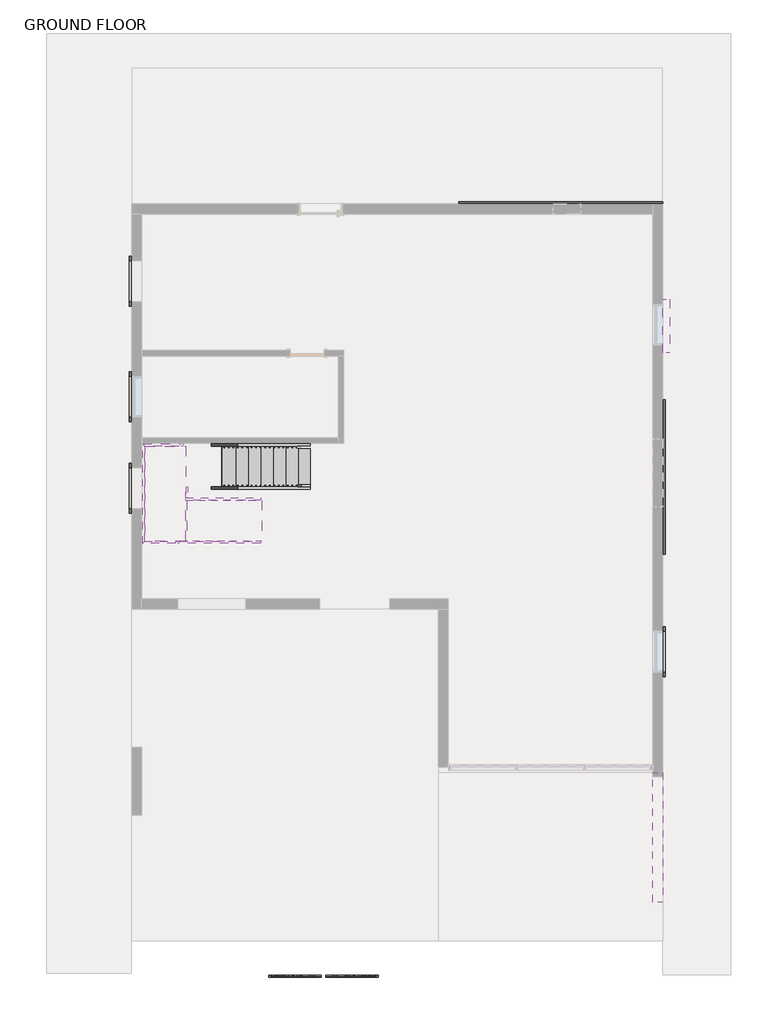
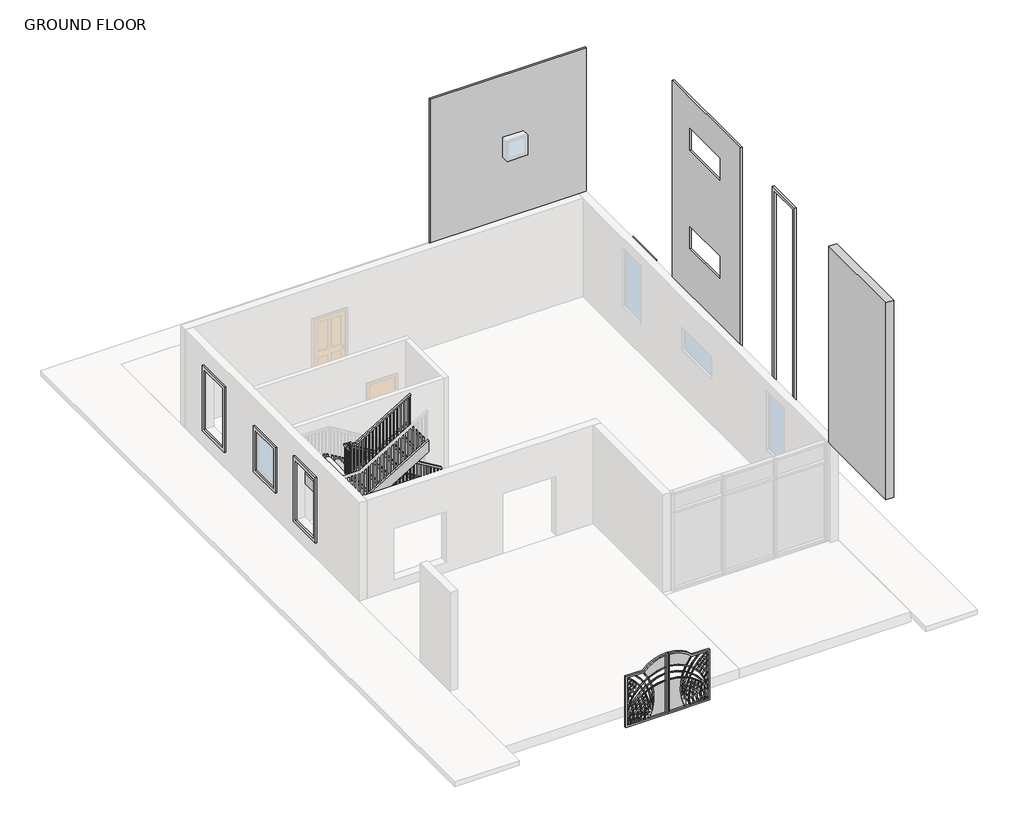
# One storey, part 3 of 3: 9 proxies, 8 members, 2 stair flights, 1 railing, 1 slab.
"""IFC4 building model written with IfcOpenShell, lengths in millimetres."""

from ifc_helpers import new_model, si_unit, frame, origin, place, context, project, spatial, polyline, outline, extrude, faceted_brep, transform, mapped, element, save
from components import generic_models_1_generic_models_1_1482fe98, generic_models_13_generic_models_13_61cfa3f2, generic_models_14_generic_models_13_4ffb657b, generic_models_17_generic_models_17_cb6d61f1, generic_models_20_generic_models_20_543834f7, generic_models_21_generic_models_23_029173b4, generic_models_24_generic_models_24_8205a677, gate_7956_gate_7956_6bc30956, non_monolithic_landing_459b2879, stair_flight_26c172ca, stair_flight_86d1b198

model = new_model("IFC4")

# Units and contexts
model_context = context("Model", 3, world=origin())
ifc_project = project(units=[si_unit("LENGTHUNIT", "METRE", prefix="MILLI")], contexts=[model_context])

# Site, building, storey
site = spatial("IfcSite", under=ifc_project)
building = spatial("IfcBuilding", under=site)
storey = spatial("IfcBuildingStorey", under=building, Name="GROUND FLOOR", Elevation=304.8)

# Proxies
placement = place(None, origin())
generic_models_1_generic_models_1_shape = generic_models_1_generic_models_1_1482fe98(model_context)
element("IfcBuildingElementProxy", 1, Name="Generic Models 1 : Generic Models 1", ObjectType="Generic Models 1 : Generic Models 1", at=placement, inside=storey, context=model_context, shape_type="MappedRepresentation", body=[
    mapped(generic_models_1_generic_models_1_shape, transform((0.0, 0.0, 0.0), x_axis=(1.0, 0.0, 0.0), y_axis=(0.0, 1.0, 0.0), z_axis=(0.0, 0.0, 1.0))),
])
generic_models_13_generic_models_13_shape = generic_models_13_generic_models_13_61cfa3f2(model_context)
element("IfcBuildingElementProxy", 2, Name="Generic Models 13 : Generic Models 13", ObjectType="Generic Models 13 : Generic Models 13", at=placement, inside=storey, context=model_context, shape_type="MappedRepresentation", body=[
    mapped(generic_models_13_generic_models_13_shape, transform((0.0, 0.0, 0.0), x_axis=(1.0, 0.0, 0.0), y_axis=(0.0, 1.0, 0.0), z_axis=(0.0, 0.0, 1.0))),
])
generic_models_14_generic_models_13_shape = generic_models_14_generic_models_13_4ffb657b(model_context)
element("IfcBuildingElementProxy", 3, Name="Generic Models 16 : Generic Models 13", ObjectType="Generic Models 16 : Generic Models 13", at=placement, inside=storey, context=model_context, shape_type="MappedRepresentation", body=[
    mapped(generic_models_14_generic_models_13_shape, transform((0.0, 7315.2, -6096.0), x_axis=(1.0, 0.0, 0.0), y_axis=(0.0, 1.0, 0.0), z_axis=(0.0, 0.0, 1.0))),
])
generic_models_17_generic_models_17_shape = generic_models_17_generic_models_17_cb6d61f1(model_context)
element("IfcBuildingElementProxy", 4, Name="Generic Models 17 : Generic Models 17", ObjectType="Generic Models 17 : Generic Models 17", at=placement, inside=storey, context=model_context, shape_type="MappedRepresentation", body=[
    mapped(generic_models_17_generic_models_17_shape, transform((0.0, 0.0, 0.0), x_axis=(1.0, 0.0, 0.0), y_axis=(0.0, 1.0, 0.0), z_axis=(0.0, 0.0, 1.0))),
])
generic_models_20_generic_models_20_shape = generic_models_20_generic_models_20_543834f7(model_context)
element("IfcBuildingElementProxy", 5, Name="Generic Models 20 : Generic Models 20", ObjectType="Generic Models 20 : Generic Models 20", at=placement, inside=storey, context=model_context, shape_type="MappedRepresentation", body=[
    mapped(generic_models_20_generic_models_20_shape, transform((0.0, 0.0, 0.0), x_axis=(1.0, 0.0, 0.0), y_axis=(0.0, 1.0, 0.0), z_axis=(0.0, 0.0, 1.0))),
])
generic_models_21_generic_models_23_shape = generic_models_21_generic_models_23_029173b4(model_context)
element("IfcBuildingElementProxy", 6, Name="Generic Models 22 : Generic Models 23", ObjectType="Generic Models 22 : Generic Models 23", at=placement, inside=storey, context=model_context, shape_type="MappedRepresentation", body=[
    mapped(generic_models_21_generic_models_23_shape, transform((0.0, 0.0, -6400.8), x_axis=(1.0, 0.0, 0.0), y_axis=(0.0, 1.0, 0.0), z_axis=(0.0, 0.0, 1.0))),
])
generic_models_24_generic_models_24_shape = generic_models_24_generic_models_24_8205a677(model_context)
element("IfcBuildingElementProxy", 7, Name="Generic Models 26 : Generic Models 24", ObjectType="Generic Models 26 : Generic Models 24", at=placement, inside=storey, context=model_context, shape_type="MappedRepresentation", body=[
    mapped(generic_models_24_generic_models_24_shape, transform((0.0, 0.0, -6096.0), x_axis=(1.0, 0.0, 0.0), y_axis=(0.0, 1.0, 0.0), z_axis=(0.0, 0.0, 1.0))),
])
element("IfcBuildingElementProxy", 8, Name="Generic Models 29 : Generic Models 23", ObjectType="Generic Models 29 : Generic Models 23", at=placement, inside=storey, context=model_context, shape_type="MappedRepresentation", body=[
    mapped(generic_models_21_generic_models_23_shape, transform((0.0, -4635.5, -6400.8), x_axis=(1.0, 0.0, 0.0), y_axis=(0.0, 1.0, 0.0), z_axis=(0.0, 0.0, 1.0))),
])
gate_7956_gate_7956_shape = gate_7956_gate_7956_6bc30956(model_context)
element("IfcBuildingElementProxy", 9, Name="gate_7956 : gate_7956", ObjectType="gate_7956 : gate_7956", at=placement, inside=storey, context=model_context, shape_type="MappedRepresentation", body=[
    mapped(gate_7956_gate_7956_shape, transform((-5706.3281265, -8922.5779205, 304.8), x_axis=(1.0, 0.0, 0.0), y_axis=(0.0, 1.0, 0.0), z_axis=(0.0, 0.0, 1.0))),
])

# Members
element("IfcMember", 10, ObjectType="Stringer - 2\" Width", at=placement, inside=storey, context=model_context, shape_type="SweptSolid", body=[
    extrude(outline(polyline([(304.8, -5990.8517085), (516.914512, -5990.8517085), (2179.4599665, -8734.0517085), (1823.051205, -8734.0517085), (304.8, -6228.9372203), (304.8, -5990.8517085)])), frame((0.0, 1953.8826226, 0.0), z_axis=(0.0, 1.0, 0.0), x_axis=(0.0, 0.0, 1.0)), (0.0, 0.0, 1.0), 50.8),
])
element("IfcMember", 11, ObjectType="Stringer - 2\" Width", at=placement, inside=storey, context=model_context, shape_type="SweptSolid", body=[
    extrude(outline(polyline([(304.8, -5990.8517085), (516.914512, -5990.8517085), (2243.6666667, -8839.9927638), (1938.8666667, -8925.1472203), (304.8, -6228.9372203), (304.8, -5990.8517085)])), frame((0.0, 2919.0826226, 0.0), z_axis=(0.0, 1.0, 0.0), x_axis=(0.0, 0.0, 1.0)), (0.0, 0.0, 1.0), 50.8),
])
element("IfcMember", 12, ObjectType="Stringer - 2\" Width", at=placement, inside=storey, context=model_context, shape_type="SweptSolid", body=[
    extrude(outline(polyline([(2379.5811786, -8784.8517085), (2023.1724171, -8784.8517085), (3039.1724171, -7108.4517085), (3395.5811786, -7108.4517085), (2379.5811786, -8784.8517085)])), frame((0.0, 1706.4165128, 0.0), z_axis=(0.0, 1.0, 0.0), x_axis=(0.0, 0.0, 1.0)), (0.0, 0.0, 1.0), 50.8),
])
element("IfcMember", 13, ObjectType="Stringer - 2\" Width", at=placement, inside=storey, context=model_context, shape_type="SweptSolid", body=[
    extrude(outline(polyline([(2243.6666667, -9009.1106533), (1938.8666667, -8923.9561967), (3039.1724171, -7108.4517085), (3395.5811786, -7108.4517085), (2243.6666667, -9009.1106533)])), frame((0.0, 741.2165128, 0.0), z_axis=(0.0, 1.0, 0.0), x_axis=(0.0, 0.0, 1.0)), (0.0, 0.0, 1.0), 50.8),
])
element("IfcMember", 14, ObjectType="Stringer - 2\" Width", at=placement, inside=storey, context=model_context, shape_type="SweptSolid", body=[
    extrude(outline(polyline([(-8734.0517085, 1757.2165128), (-8784.8517085, 1757.2165128), (-8784.8517085, 2004.6826226), (-8734.0517085, 2004.6826226), (-8734.0517085, 1757.2165128)])), frame((0.0, 0.0, 1938.8666667), z_axis=(0.0, 0.0, 1.0), x_axis=(1.0, 0.0, 0.0)), (0.0, 0.0, 1.0), 304.8),
])
element("IfcMember", 15, ObjectType="Stringer - 2\" Width", at=placement, inside=storey, context=model_context, shape_type="Brep", body=[
    faceted_brep([(-8839.9927638, 2919.0826226, 2243.6666667), (-8839.9927638, 2969.8826226, 2243.6666667), (-9750.0517085, 2969.8826226, 2243.6666667), (-9699.2517085, 2919.0826226, 2243.6666667), (-8925.1472203, 2919.0826226, 1938.8666667), (-9699.2517085, 2919.0826226, 1938.8666667), (-8925.1472203, 2969.8826226, 1938.8666667), (-9750.0517085, 2969.8826226, 1938.8666667)], [[[0, 1, 2, 3]], [[4, 0, 3, 5]], [[6, 4, 5, 7]], [[1, 6, 7, 2]], [[1, 0, 4, 6]], [[2, 7, 5, 3]]]),
])
element("IfcMember", 16, ObjectType="Stringer - 2\" Width", at=placement, inside=storey, context=model_context, shape_type="SweptSolid", body=[
    extrude(outline(polyline([(-9750.0517085, 2969.8826226), (-9699.2517085, 2919.0826226), (-9699.2517085, 792.0165128), (-9750.0517085, 741.2165128), (-9750.0517085, 2969.8826226)])), frame((0.0, 0.0, 1938.8666667), z_axis=(0.0, 0.0, 1.0), x_axis=(1.0, 0.0, 0.0)), (0.0, 0.0, 1.0), 304.8),
])
element("IfcMember", 17, ObjectType="Stringer - 2\" Width", at=placement, inside=storey, context=model_context, shape_type="Brep", body=[
    faceted_brep([(-9699.2517085, 792.0165128, 2243.6666667), (-9750.0517085, 741.2165128, 2243.6666667), (-9009.1106533, 741.2165128, 2243.6666667), (-9009.1106533, 792.0165128, 2243.6666667), (-9699.2517085, 792.0165128, 1938.8666667), (-8923.9561967, 792.0165128, 1938.8666667), (-9750.0517085, 741.2165128, 1938.8666667), (-8923.9561967, 741.2165128, 1938.8666667)], [[[0, 1, 2, 3]], [[4, 0, 3, 5]], [[6, 4, 5, 7]], [[1, 6, 7, 2]], [[1, 0, 4, 6]], [[2, 7, 5, 3]]]),
])

# Railing
element("IfcRailing", 18, ObjectType="Handrail - Rectangular", at=placement, inside=storey, context=model_context, shape_type="SolidModel", body=[
    faceted_brep([(-5990.8517085, 2004.6826226, 1388.5333333), (-5990.8517085, 2004.6826226, 1329.1318731), (-5990.8517085, 2055.4826226, 1329.1318731), (-5990.8517085, 2055.4826226, 1388.5333333), (-8708.6517085, 2004.6826226, 3035.6848485), (-8759.4517085, 2004.6826226, 3007.071267), (-8759.4517085, 2055.4826226, 3007.071267), (-8708.6517085, 2055.4826226, 3035.6848485), (-8708.6517085, 2004.6826226, 3081.8666667), (-8759.4517085, 2004.6826226, 3031.0666667), (-8759.4517085, 2055.4826226, 3031.0666667), (-8708.6517085, 2055.4826226, 3081.8666667), (-8784.8517085, 2004.6826226, 3081.8666667), (-8784.8517085, 2004.6826226, 3031.0666667), (-8835.6517085, 2055.4826226, 3031.0666667), (-8835.6517085, 2055.4826226, 3081.8666667), (-8784.8517085, 1928.4826226, 3081.8666667), (-8784.8517085, 1928.4826226, 3031.0666667), (-8835.6517085, 1928.4826226, 3031.0666667), (-8835.6517085, 1928.4826226, 3081.8666667), (-8784.8517085, 1782.6165128, 3081.8666667), (-8784.8517085, 1731.8165128, 3031.0666667), (-8835.6517085, 1731.8165128, 3031.0666667), (-8835.6517085, 1782.6165128, 3081.8666667), (-8784.8517085, 1782.6165128, 3297.3818182), (-8784.8517085, 1731.8165128, 3246.5818182), (-8835.6517085, 1731.8165128, 3246.5818182), (-8835.6517085, 1782.6165128, 3297.3818182), (-8784.8517085, 1706.4165128, 3297.3818182), (-8784.8517085, 1706.4165128, 3246.5818182), (-8835.6517085, 1655.6165128, 3246.5818182), (-8835.6517085, 1655.6165128, 3297.3818182), (-8708.6517085, 1706.4165128, 3297.3818182), (-8694.4592991, 1706.4165128, 3246.5818182), (-8694.4592991, 1655.6165128, 3246.5818182), (-8708.6517085, 1655.6165128, 3297.3818182), (-7108.4517085, 1706.4165128, 4267.2), (-7108.4517085, 1655.6165128, 4267.2), (-7108.4517085, 1655.6165128, 4207.7985397), (-7108.4517085, 1706.4165128, 4207.7985397)], [[[0, 1, 2, 3]], [[1, 0, 4, 5]], [[2, 1, 5, 6]], [[3, 2, 6, 7]], [[0, 3, 7, 4]], [[5, 4, 8, 9]], [[6, 5, 9, 10]], [[7, 6, 10, 11]], [[4, 7, 11, 8]], [[9, 8, 12, 13]], [[10, 9, 13, 14]], [[11, 10, 14, 15]], [[8, 11, 15, 12]], [[13, 12, 16, 17]], [[14, 13, 17, 18]], [[15, 14, 18, 19]], [[12, 15, 19, 16]], [[17, 16, 20, 21]], [[18, 17, 21, 22]], [[19, 18, 22, 23]], [[16, 19, 23, 20]], [[21, 20, 24, 25]], [[22, 21, 25, 26]], [[23, 22, 26, 27]], [[20, 23, 27, 24]], [[25, 24, 28, 29]], [[26, 25, 29, 30]], [[27, 26, 30, 31]], [[24, 27, 31, 28]], [[29, 28, 32, 33]], [[30, 29, 33, 34]], [[31, 30, 34, 35]], [[28, 31, 35, 32]], [[36, 37, 38, 39]], [[33, 32, 36, 39]], [[34, 33, 39, 38]], [[35, 34, 38, 37]], [[32, 35, 37, 36]]]),
    extrude(outline(polyline([(4155.8439943, -7194.1767085), (3183.4666667, -7194.1767085), (3183.4666667, -7175.1267085), (4167.3894488, -7175.1267085), (4155.8439943, -7194.1767085)])), frame((0.0, 1671.4915128, 0.0), z_axis=(0.0, 1.0, 0.0), x_axis=(0.0, 0.0, 1.0)), (0.0, 0.0, 1.0), 19.05),
    extrude(outline(polyline([(4094.2682367, -7295.7767085), (3183.4666667, -7295.7767085), (3183.4666667, -7276.7267085), (4105.8136913, -7276.7267085), (4094.2682367, -7295.7767085)])), frame((0.0, 1671.4915128, 0.0), z_axis=(0.0, 1.0, 0.0), x_axis=(0.0, 0.0, 1.0)), (0.0, 0.0, 1.0), 19.05),
    extrude(outline(polyline([(4032.6924791, -7397.3767085), (3183.4666667, -7397.3767085), (3183.4666667, -7378.3267085), (4044.2379337, -7378.3267085), (4032.6924791, -7397.3767085)])), frame((0.0, 1671.4915128, 0.0), z_axis=(0.0, 1.0, 0.0), x_axis=(0.0, 0.0, 1.0)), (0.0, 0.0, 1.0), 19.05),
    extrude(outline(polyline([(3971.1167216, -7498.9767085), (3014.1333333, -7498.9767085), (3014.1333333, -7479.9267085), (3982.6621761, -7479.9267085), (3971.1167216, -7498.9767085)])), frame((0.0, 1671.4915128, 0.0), z_axis=(0.0, 1.0, 0.0), x_axis=(0.0, 0.0, 1.0)), (0.0, 0.0, 1.0), 19.05),
    extrude(outline(polyline([(3909.540964, -7600.5767085), (3014.1333333, -7600.5767085), (3014.1333333, -7581.5267085), (3921.0864185, -7581.5267085), (3909.540964, -7600.5767085)])), frame((0.0, 1671.4915128, 0.0), z_axis=(0.0, 1.0, 0.0), x_axis=(0.0, 0.0, 1.0)), (0.0, 0.0, 1.0), 19.05),
    extrude(outline(polyline([(3847.9652064, -7702.1767085), (2844.8, -7702.1767085), (2844.8, -7683.1267085), (3859.510661, -7683.1267085), (3847.9652064, -7702.1767085)])), frame((0.0, 1671.4915128, 0.0), z_axis=(0.0, 1.0, 0.0), x_axis=(0.0, 0.0, 1.0)), (0.0, 0.0, 1.0), 19.05),
    extrude(outline(polyline([(3786.3894488, -7803.7767085), (2844.8, -7803.7767085), (2844.8, -7784.7267085), (3797.9349034, -7784.7267085), (3786.3894488, -7803.7767085)])), frame((0.0, 1671.4915128, 0.0), z_axis=(0.0, 1.0, 0.0), x_axis=(0.0, 0.0, 1.0)), (0.0, 0.0, 1.0), 19.05),
    extrude(outline(polyline([(3724.8136913, -7905.3767085), (2844.8, -7905.3767085), (2844.8, -7886.3267085), (3736.3591458, -7886.3267085), (3724.8136913, -7905.3767085)])), frame((0.0, 1671.4915128, 0.0), z_axis=(0.0, 1.0, 0.0), x_axis=(0.0, 0.0, 1.0)), (0.0, 0.0, 1.0), 19.05),
    extrude(outline(polyline([(3663.2379337, -8006.9767085), (2675.4666667, -8006.9767085), (2675.4666667, -7987.9267085), (3674.7833882, -7987.9267085), (3663.2379337, -8006.9767085)])), frame((0.0, 1671.4915128, 0.0), z_axis=(0.0, 1.0, 0.0), x_axis=(0.0, 0.0, 1.0)), (0.0, 0.0, 1.0), 19.05),
    extrude(outline(polyline([(3601.6621761, -8108.5767085), (2675.4666667, -8108.5767085), (2675.4666667, -8089.5267085), (3613.2076307, -8089.5267085), (3601.6621761, -8108.5767085)])), frame((0.0, 1671.4915128, 0.0), z_axis=(0.0, 1.0, 0.0), x_axis=(0.0, 0.0, 1.0)), (0.0, 0.0, 1.0), 19.05),
    extrude(outline(polyline([(3540.0864185, -8210.1767085), (2675.4666667, -8210.1767085), (2675.4666667, -8191.1267085), (3551.6318731, -8191.1267085), (3540.0864185, -8210.1767085)])), frame((0.0, 1671.4915128, 0.0), z_axis=(0.0, 1.0, 0.0), x_axis=(0.0, 0.0, 1.0)), (0.0, 0.0, 1.0), 19.05),
    extrude(outline(polyline([(3478.510661, -8311.7767085), (2506.1333333, -8311.7767085), (2506.1333333, -8292.7267085), (3490.0561155, -8292.7267085), (3478.510661, -8311.7767085)])), frame((0.0, 1671.4915128, 0.0), z_axis=(0.0, 1.0, 0.0), x_axis=(0.0, 0.0, 1.0)), (0.0, 0.0, 1.0), 19.05),
    extrude(outline(polyline([(3416.9349034, -8413.3767085), (2506.1333333, -8413.3767085), (2506.1333333, -8394.3267085), (3428.4803579, -8394.3267085), (3416.9349034, -8413.3767085)])), frame((0.0, 1671.4915128, 0.0), z_axis=(0.0, 1.0, 0.0), x_axis=(0.0, 0.0, 1.0)), (0.0, 0.0, 1.0), 19.05),
    extrude(outline(polyline([(3355.3591458, -8514.9767085), (2506.1333333, -8514.9767085), (2506.1333333, -8495.9267085), (3366.9046004, -8495.9267085), (3355.3591458, -8514.9767085)])), frame((0.0, 1671.4915128, 0.0), z_axis=(0.0, 1.0, 0.0), x_axis=(0.0, 0.0, 1.0)), (0.0, 0.0, 1.0), 19.05),
    extrude(outline(polyline([(3293.7833882, -8616.5767085), (2336.8, -8616.5767085), (2336.8, -8597.5267085), (3305.3288428, -8597.5267085), (3293.7833882, -8616.5767085)])), frame((0.0, 1671.4915128, 0.0), z_axis=(0.0, 1.0, 0.0), x_axis=(0.0, 0.0, 1.0)), (0.0, 0.0, 1.0), 19.05),
    extrude(outline(polyline([(3232.2076307, -8718.1767085), (2336.8, -8718.1767085), (2336.8, -8699.1267085), (3243.7530852, -8699.1267085), (3232.2076307, -8718.1767085)])), frame((0.0, 1671.4915128, 0.0), z_axis=(0.0, 1.0, 0.0), x_axis=(0.0, 0.0, 1.0)), (0.0, 0.0, 1.0), 19.05),
    extrude(outline(polyline([(-8800.7267085, 1734.8076226), (-8800.7267085, 1715.7576226), (-8819.7767085, 1715.7576226), (-8819.7767085, 1734.8076226), (-8800.7267085, 1734.8076226)])), frame((0.0, 0.0, 2167.4666667), z_axis=(0.0, 0.0, 1.0), x_axis=(1.0, 0.0, 0.0)), (0.0, 0.0, 1.0), 1079.1151515),
    extrude(outline(polyline([(-8800.7267085, 1836.4076226), (-8800.7267085, 1817.3576226), (-8819.7767085, 1817.3576226), (-8819.7767085, 1836.4076226), (-8800.7267085, 1836.4076226)])), frame((0.0, 0.0, 2167.4666667), z_axis=(0.0, 0.0, 1.0), x_axis=(1.0, 0.0, 0.0)), (0.0, 0.0, 1.0), 863.6),
    extrude(outline(polyline([(-8800.7267085, 1938.0076226), (-8800.7267085, 1918.9576226), (-8819.7767085, 1918.9576226), (-8819.7767085, 1938.0076226), (-8800.7267085, 1938.0076226)])), frame((0.0, 0.0, 2167.4666667), z_axis=(0.0, 0.0, 1.0), x_axis=(1.0, 0.0, 0.0)), (0.0, 0.0, 1.0), 863.6),
    extrude(outline(polyline([(-8724.5267085, 2020.5576226), (-8743.5767085, 2020.5576226), (-8743.5767085, 2039.6076226), (-8724.5267085, 2039.6076226), (-8724.5267085, 2020.5576226)])), frame((0.0, 0.0, 1998.1333333), z_axis=(0.0, 0.0, 1.0), x_axis=(1.0, 0.0, 0.0)), (0.0, 0.0, 1.0), 1032.9333333),
    extrude(outline(polyline([(2935.8742973, -8641.9767085), (1998.1333333, -8641.9767085), (1998.1333333, -8622.9267085), (2924.3288428, -8622.9267085), (2935.8742973, -8641.9767085)])), frame((0.0, 2020.5576226, 0.0), z_axis=(0.0, 1.0, 0.0), x_axis=(0.0, 0.0, 1.0)), (0.0, 0.0, 1.0), 19.05),
    extrude(outline(polyline([(2874.2985397, -8540.3767085), (1998.1333333, -8540.3767085), (1998.1333333, -8521.3267085), (2862.7530852, -8521.3267085), (2874.2985397, -8540.3767085)])), frame((0.0, 2020.5576226, 0.0), z_axis=(0.0, 1.0, 0.0), x_axis=(0.0, 0.0, 1.0)), (0.0, 0.0, 1.0), 19.05),
    extrude(outline(polyline([(2812.7227822, -8438.7767085), (1828.8, -8438.7767085), (1828.8, -8419.7267085), (2801.1773276, -8419.7267085), (2812.7227822, -8438.7767085)])), frame((0.0, 2020.5576226, 0.0), z_axis=(0.0, 1.0, 0.0), x_axis=(0.0, 0.0, 1.0)), (0.0, 0.0, 1.0), 19.05),
    extrude(outline(polyline([(2751.1470246, -8337.1767085), (1828.8, -8337.1767085), (1828.8, -8318.1267085), (2739.60157, -8318.1267085), (2751.1470246, -8337.1767085)])), frame((0.0, 2020.5576226, 0.0), z_axis=(0.0, 1.0, 0.0), x_axis=(0.0, 0.0, 1.0)), (0.0, 0.0, 1.0), 19.05),
    extrude(outline(polyline([(2689.571267, -8235.5767085), (1828.8, -8235.5767085), (1828.8, -8216.5267085), (2678.0258125, -8216.5267085), (2689.571267, -8235.5767085)])), frame((0.0, 2020.5576226, 0.0), z_axis=(0.0, 1.0, 0.0), x_axis=(0.0, 0.0, 1.0)), (0.0, 0.0, 1.0), 19.05),
    extrude(outline(polyline([(2627.9955094, -8133.9767085), (1659.4666667, -8133.9767085), (1659.4666667, -8114.9267085), (2616.4500549, -8114.9267085), (2627.9955094, -8133.9767085)])), frame((0.0, 2020.5576226, 0.0), z_axis=(0.0, 1.0, 0.0), x_axis=(0.0, 0.0, 1.0)), (0.0, 0.0, 1.0), 19.05),
    extrude(outline(polyline([(2566.4197519, -8032.3767085), (1659.4666667, -8032.3767085), (1659.4666667, -8013.3267085), (2554.8742973, -8013.3267085), (2566.4197519, -8032.3767085)])), frame((0.0, 2020.5576226, 0.0), z_axis=(0.0, 1.0, 0.0), x_axis=(0.0, 0.0, 1.0)), (0.0, 0.0, 1.0), 19.05),
    extrude(outline(polyline([(2504.8439943, -7930.7767085), (1490.1333333, -7930.7767085), (1490.1333333, -7911.7267085), (2493.2985397, -7911.7267085), (2504.8439943, -7930.7767085)])), frame((0.0, 2020.5576226, 0.0), z_axis=(0.0, 1.0, 0.0), x_axis=(0.0, 0.0, 1.0)), (0.0, 0.0, 1.0), 19.05),
    extrude(outline(polyline([(2443.2682367, -7829.1767085), (1490.1333333, -7829.1767085), (1490.1333333, -7810.1267085), (2431.7227822, -7810.1267085), (2443.2682367, -7829.1767085)])), frame((0.0, 2020.5576226, 0.0), z_axis=(0.0, 1.0, 0.0), x_axis=(0.0, 0.0, 1.0)), (0.0, 0.0, 1.0), 19.05),
    extrude(outline(polyline([(2381.6924791, -7727.5767085), (1490.1333333, -7727.5767085), (1490.1333333, -7708.5267085), (2370.1470246, -7708.5267085), (2381.6924791, -7727.5767085)])), frame((0.0, 2020.5576226, 0.0), z_axis=(0.0, 1.0, 0.0), x_axis=(0.0, 0.0, 1.0)), (0.0, 0.0, 1.0), 19.05),
    extrude(outline(polyline([(2320.1167216, -7625.9767085), (1320.8, -7625.9767085), (1320.8, -7606.9267085), (2308.571267, -7606.9267085), (2320.1167216, -7625.9767085)])), frame((0.0, 2020.5576226, 0.0), z_axis=(0.0, 1.0, 0.0), x_axis=(0.0, 0.0, 1.0)), (0.0, 0.0, 1.0), 19.05),
    extrude(outline(polyline([(2258.540964, -7524.3767085), (1320.8, -7524.3767085), (1320.8, -7505.3267085), (2246.9955094, -7505.3267085), (2258.540964, -7524.3767085)])), frame((0.0, 2020.5576226, 0.0), z_axis=(0.0, 1.0, 0.0), x_axis=(0.0, 0.0, 1.0)), (0.0, 0.0, 1.0), 19.05),
    extrude(outline(polyline([(2196.9652064, -7422.7767085), (1320.8, -7422.7767085), (1320.8, -7403.7267085), (2185.4197519, -7403.7267085), (2196.9652064, -7422.7767085)])), frame((0.0, 2020.5576226, 0.0), z_axis=(0.0, 1.0, 0.0), x_axis=(0.0, 0.0, 1.0)), (0.0, 0.0, 1.0), 19.05),
    extrude(outline(polyline([(2135.3894488, -7321.1767085), (1151.4666667, -7321.1767085), (1151.4666667, -7302.1267085), (2123.8439943, -7302.1267085), (2135.3894488, -7321.1767085)])), frame((0.0, 2020.5576226, 0.0), z_axis=(0.0, 1.0, 0.0), x_axis=(0.0, 0.0, 1.0)), (0.0, 0.0, 1.0), 19.05),
    extrude(outline(polyline([(2073.8136913, -7219.5767085), (1151.4666667, -7219.5767085), (1151.4666667, -7200.5267085), (2062.2682367, -7200.5267085), (2073.8136913, -7219.5767085)])), frame((0.0, 2020.5576226, 0.0), z_axis=(0.0, 1.0, 0.0), x_axis=(0.0, 0.0, 1.0)), (0.0, 0.0, 1.0), 19.05),
    extrude(outline(polyline([(2012.2379337, -7117.9767085), (1151.4666667, -7117.9767085), (1151.4666667, -7098.9267085), (2000.6924791, -7098.9267085), (2012.2379337, -7117.9767085)])), frame((0.0, 2020.5576226, 0.0), z_axis=(0.0, 1.0, 0.0), x_axis=(0.0, 0.0, 1.0)), (0.0, 0.0, 1.0), 19.05),
    extrude(outline(polyline([(1950.6621761, -7016.3767085), (982.1333333, -7016.3767085), (982.1333333, -6997.3267085), (1939.1167216, -6997.3267085), (1950.6621761, -7016.3767085)])), frame((0.0, 2020.5576226, 0.0), z_axis=(0.0, 1.0, 0.0), x_axis=(0.0, 0.0, 1.0)), (0.0, 0.0, 1.0), 19.05),
    extrude(outline(polyline([(1889.0864185, -6914.7767085), (982.1333333, -6914.7767085), (982.1333333, -6895.7267085), (1877.540964, -6895.7267085), (1889.0864185, -6914.7767085)])), frame((0.0, 2020.5576226, 0.0), z_axis=(0.0, 1.0, 0.0), x_axis=(0.0, 0.0, 1.0)), (0.0, 0.0, 1.0), 19.05),
    extrude(outline(polyline([(1827.510661, -6813.1767085), (812.8, -6813.1767085), (812.8, -6794.1267085), (1815.9652064, -6794.1267085), (1827.510661, -6813.1767085)])), frame((0.0, 2020.5576226, 0.0), z_axis=(0.0, 1.0, 0.0), x_axis=(0.0, 0.0, 1.0)), (0.0, 0.0, 1.0), 19.05),
    extrude(outline(polyline([(1765.9349034, -6711.5767085), (812.8, -6711.5767085), (812.8, -6692.5267085), (1754.3894488, -6692.5267085), (1765.9349034, -6711.5767085)])), frame((0.0, 2020.5576226, 0.0), z_axis=(0.0, 1.0, 0.0), x_axis=(0.0, 0.0, 1.0)), (0.0, 0.0, 1.0), 19.05),
    extrude(outline(polyline([(1704.3591458, -6609.9767085), (812.8, -6609.9767085), (812.8, -6590.9267085), (1692.8136913, -6590.9267085), (1704.3591458, -6609.9767085)])), frame((0.0, 2020.5576226, 0.0), z_axis=(0.0, 1.0, 0.0), x_axis=(0.0, 0.0, 1.0)), (0.0, 0.0, 1.0), 19.05),
    extrude(outline(polyline([(1642.7833882, -6508.3767085), (643.4666667, -6508.3767085), (643.4666667, -6489.3267085), (1631.2379337, -6489.3267085), (1642.7833882, -6508.3767085)])), frame((0.0, 2020.5576226, 0.0), z_axis=(0.0, 1.0, 0.0), x_axis=(0.0, 0.0, 1.0)), (0.0, 0.0, 1.0), 19.05),
    extrude(outline(polyline([(1581.2076307, -6406.7767085), (643.4666667, -6406.7767085), (643.4666667, -6387.7267085), (1569.6621761, -6387.7267085), (1581.2076307, -6406.7767085)])), frame((0.0, 2020.5576226, 0.0), z_axis=(0.0, 1.0, 0.0), x_axis=(0.0, 0.0, 1.0)), (0.0, 0.0, 1.0), 19.05),
    extrude(outline(polyline([(1519.6318731, -6305.1767085), (643.4666667, -6305.1767085), (643.4666667, -6286.1267085), (1508.0864185, -6286.1267085), (1519.6318731, -6305.1767085)])), frame((0.0, 2020.5576226, 0.0), z_axis=(0.0, 1.0, 0.0), x_axis=(0.0, 0.0, 1.0)), (0.0, 0.0, 1.0), 19.05),
    extrude(outline(polyline([(1458.0561155, -6203.5767085), (474.1333333, -6203.5767085), (474.1333333, -6184.5267085), (1446.510661, -6184.5267085), (1458.0561155, -6203.5767085)])), frame((0.0, 2020.5576226, 0.0), z_axis=(0.0, 1.0, 0.0), x_axis=(0.0, 0.0, 1.0)), (0.0, 0.0, 1.0), 19.05),
    extrude(outline(polyline([(1396.4803579, -6101.9767085), (474.1333333, -6101.9767085), (474.1333333, -6082.9267085), (1384.9349034, -6082.9267085), (1396.4803579, -6101.9767085)])), frame((0.0, 2020.5576226, 0.0), z_axis=(0.0, 1.0, 0.0), x_axis=(0.0, 0.0, 1.0)), (0.0, 0.0, 1.0), 19.05),
    extrude(outline(polyline([(-8800.7267085, 1690.5415128), (-8800.7267085, 1671.4915128), (-8819.7767085, 1671.4915128), (-8819.7767085, 1690.5415128), (-8800.7267085, 1690.5415128)])), frame((0.0, 0.0, 2167.4666667), z_axis=(0.0, 0.0, 1.0), x_axis=(1.0, 0.0, 0.0)), (0.0, 0.0, 1.0), 1079.1151515),
    extrude(outline(polyline([(-8800.7267085, 2020.5576226), (-8819.7767085, 2020.5576226), (-8819.7767085, 2039.6076226), (-8800.7267085, 2039.6076226), (-8800.7267085, 2020.5576226)])), frame((0.0, 0.0, 2167.4666667), z_axis=(0.0, 0.0, 1.0), x_axis=(1.0, 0.0, 0.0)), (0.0, 0.0, 1.0), 863.6),
    extrude(outline(polyline([(4196.2530852, -7127.5017085), (3183.4666667, -7127.5017085), (3183.4666667, -7108.4517085), (4207.7985397, -7108.4517085), (4196.2530852, -7127.5017085)])), frame((0.0, 1671.4915128, 0.0), z_axis=(0.0, 1.0, 0.0), x_axis=(0.0, 0.0, 1.0)), (0.0, 0.0, 1.0), 19.05),
    extrude(outline(polyline([(1340.6773276, -6009.9017085), (474.1333333, -6009.9017085), (474.1333333, -5990.8517085), (1329.1318731, -5990.8517085), (1340.6773276, -6009.9017085)])), frame((0.0, 2020.5576226, 0.0), z_axis=(0.0, 1.0, 0.0), x_axis=(0.0, 0.0, 1.0)), (0.0, 0.0, 1.0), 19.05),
])

# Slab
non_monolithic_landing_shape = non_monolithic_landing_459b2879(model_context)
element("IfcSlab", 19, ObjectType="Non-Monolithic Landing", at=placement, inside=storey, context=model_context, shape_type="MappedRepresentation", body=[
    mapped(non_monolithic_landing_shape, transform((0.0, 0.0, 0.0), x_axis=(1.0, 0.0, 0.0), y_axis=(0.0, 1.0, 0.0), z_axis=(0.0, 0.0, 1.0))),
])

# Stair flights
stair_flight_shape = stair_flight_26c172ca(model_context)
element("IfcStairFlight", 20, ObjectType="2\" Tread 1\" Nosing 1/4\" Riser", at=placement, inside=storey, context=model_context, shape_type="MappedRepresentation", body=[
    mapped(stair_flight_shape, transform((0.0, 0.0, 0.0), x_axis=(1.0, 0.0, 0.0), y_axis=(0.0, 1.0, 0.0), z_axis=(0.0, 0.0, 1.0))),
])
stair_flight_2_shape = stair_flight_86d1b198(model_context)
element("IfcStairFlight", 21, ObjectType="2\" Tread 1\" Nosing 1/4\" Riser", at=placement, inside=storey, context=model_context, shape_type="MappedRepresentation", body=[
    mapped(stair_flight_2_shape, transform((0.0, 0.0, 0.0), x_axis=(1.0, 0.0, 0.0), y_axis=(0.0, 1.0, 0.0), z_axis=(0.0, 0.0, 1.0))),
])

save(model, "model.ifc")

# Revit data of these elements
# Type "gate_7956 : gate_7956"
#   m.s. sheet = none
#   2" x2" pipe = none
#   1"x1"pipe = none
#   Default Elevation = 0
# Type "Handrail - Rectangular"
#   Assembly Code = "C2010400"
#   built-in parameter 1008612 = 0.0416667 (stored number, unit not read)
#   built-in parameter 1008611 = 0.0416667 (stored number, unit not read)
#   built-in parameter 1008609 = 0.333333 (stored number, unit not read)
#   built-in parameter 1008604 = 0.166667 (stored number, unit not read)
#   built-in parameter 1008603 = 0.166667 (stored number, unit not read)
#   Railing Height = 3' - 0"
#   built-in parameter 1008630 = 2
#   built-in parameter 1008610 = 2
#   built-in parameter 1008618 = Baluster - Square : 3/4"
# Element 1 (IfcBuildingElementProxy, "Generic Models 1 : Generic Models 1")
#   Phase Created = New Construction
#   Materials on its faces: "WALL PAINT"
# Element 2 (IfcBuildingElementProxy, "Generic Models 13 : Generic Models 13")
#   Phase Created = New Construction
# Element 3 (IfcBuildingElementProxy, "Generic Models 16 : Generic Models 13")
#   Phase Created = New Construction
# Element 4 (IfcBuildingElementProxy, "Generic Models 17 : Generic Models 17")
#   Phase Created = New Construction
# Element 5 (IfcBuildingElementProxy, "Generic Models 20 : Generic Models 20")
#   Phase Created = New Construction
#   Materials on its faces: "GOLD COLOUR"
# Element 6 (IfcBuildingElementProxy, "Generic Models 22 : Generic Models 23")
#   Phase Created = New Construction
# Element 7 (IfcBuildingElementProxy, "Generic Models 26 : Generic Models 24")
#   Phase Created = New Construction
# Element 8 (IfcBuildingElementProxy, "Generic Models 29 : Generic Models 23")
#   Phase Created = New Construction
# Element 9 (IfcBuildingElementProxy, "gate_7956 : gate_7956")
#   Phase Created = New Construction
#   Materials on its faces: "r1"
# Elements 10, 11, 12, 13, 14, 15, 16, 17 (IfcMember, "Stringer - 2\" Width")
#   Phase Created = New Construction
# Element 18 (IfcRailing, "Handrail - Rectangular")
#   Phase Created = New Construction
# Element 19 (IfcSlab, "Non-Monolithic Landing")
#   Phase Created = New Construction
# Elements 20, 21 (IfcStairFlight, "2\" Tread 1\" Nosing 1/4\" Riser")
#   Phase Created = New Construction
# Materials
#   "WALL PAINT": class "Generic", colour RGB 120 120 120, transparency 0, Cost = 0
#   "GOLD COLOUR": class "Generic", colour RGB 120 120 120, transparency 0, Cost = 0
#   "r1": class "Generic", colour RGB 120 120 120, transparency 0, Cost = 0
